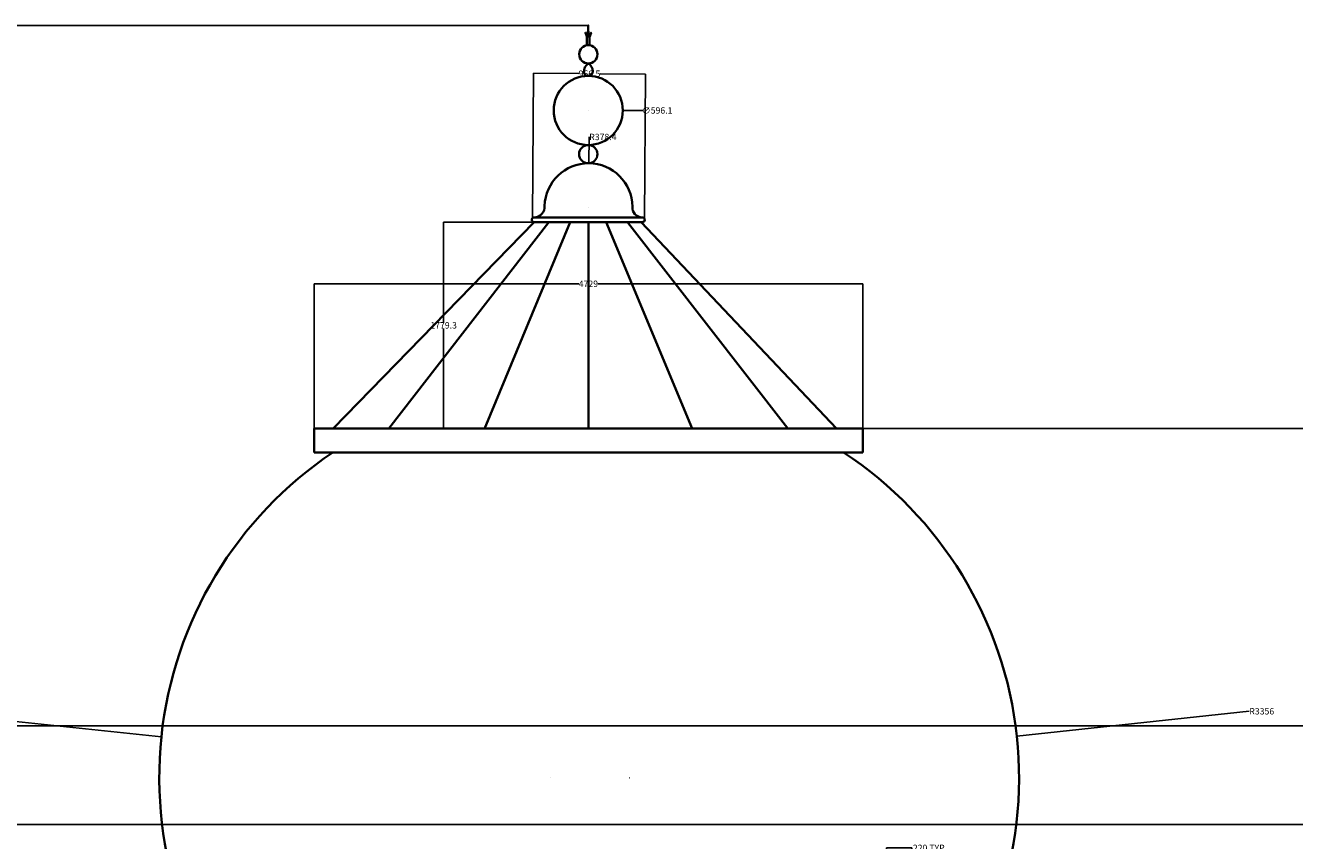
# Model space of a CAD drawing. Units: millimetres. Extents: x 8570 to 49085, y 3782 to 24863.
# Tile 10 of 15: x 17549 to 28488, y 17835 to 24863. Entities that reach past the tile are written whole.
import ezdxf

# ---------------------------------------------------------------- set-up
doc = ezdxf.new("R2010")
doc.units = ezdxf.units.MM
doc.header["$MEASUREMENT"] = 0
doc.header["$PDMODE"] = 3
doc.layers.add('A-ANNO-DIMS', color=2, linetype='Continuous', lineweight=18)
doc.layers.add('A-ROOF-DOME', color=7, linetype='Continuous', lineweight=35)
doc.styles.get("Standard").update_dxf_attribs({"font": 'arial.ttf'})
doc.dimstyles.get("Standard").update_dxf_attribs({"dimtxt": 55, "dimasz": 0.18, "dimexe": 0.18, "dimexo": 0.0625, "dimgap": 0.09, "dimtad": 0, "dimtih": 1, "dimtoh": 1, "dimdec": 0, "dimzin": 0, "dimdsep": 46, "dimtxsty": 'Standard', "dimcen": 0.09, "dimadec": 0, "dimazin": 0, "dimtfac": 1, "dimtdec": 0, "dimtofl": 0, "dimtmove": 0, "dimatfit": 3, "dimfxl": 1, "dimtolj": 1, "dimtzin": 0, "dimarcsym": 0})

# ---------------------------------------------------------------- blocks, each defined once
blk = doc.blocks.new('*D20')
at = {"layer": 'A-ANNO-DIMS', "color": 0, "lineweight": -2, "transparency": 16777216}
for p, q in [((24969, 16396.42408182047), (24969, 17772.62081909354)), ((24969.18, 17772.44081909354), (25188.82, 17772.44081909354)), ((25189, 16396.42408182047), (25189, 17772.62081909354)), ((25189, 17772.44081909354), (25189.18, 17772.44081909354))]:
    blk.add_line(p, q, dxfattribs=at)
at = {"layer": 'A-ANNO-DIMS', "color": 0, "transparency": 16777216}
for points in [[(24969.18, 17772.47081909354), (24969.18, 17772.41081909354), (24969, 17772.44081909354)], [(25188.82, 17772.47081909354), (25188.82, 17772.41081909354), (25189, 17772.44081909354)]]:
    blk.add_solid(points, dxfattribs=at)
at = {"layer": 'Defpoints', "color": 0, "transparency": 16777216}
for p in [(25189, 17772.44081909354), (24969, 16396.36158182047), (25189, 16396.36158182047)]:
    blk.add_point(p, dxfattribs=at)
at = {"layer": 'A-ANNO-DIMS', "color": 0, "transparency": 16777216, "insert": (25344.96577080491, 17772.44081909354), "char_height": 55, "attachment_point": 5}
blk.add_mtext('\\A1;220 TYP.', dxfattribs=at)
blk = doc.blocks.new('*D44')
at = {"layer": 'A-ANNO-DIMS', "color": 0, "lineweight": -2, "transparency": 16777216}
for p, q in [((22399.68750000001, 24862.95258900002), (8684.320000000003, 24862.95258900002)), ((8684.500000000005, 24862.77258900002), (8684.500000000005, 15410.3978088247)), ((8684.50000000001, 5901.680000000001), (8684.500000000005, 15354.05478017531)), ((10843.9375, 5901.500000000002), (8684.32000000001, 5901.500000000001))]:
    blk.add_line(p, q, dxfattribs=at)
at = {"layer": 'A-ANNO-DIMS', "color": 0, "transparency": 16777216}
for points in [[(8684.470000000005, 24862.77258900002), (8684.530000000006, 24862.77258900002), (8684.500000000005, 24862.95258900002)], [(8684.470000000008, 5901.680000000001), (8684.53000000001, 5901.680000000001), (8684.50000000001, 5901.500000000001)]]:
    blk.add_solid(points, dxfattribs=at)
at = {"layer": 'Defpoints', "color": 0, "transparency": 16777216}
for p in [(8684.500000000005, 24862.95258900002), (22399.75000000001, 24862.95258900002), (10844, 5901.500000000002)]:
    blk.add_point(p, dxfattribs=at)
at = {"layer": 'A-ANNO-DIMS', "color": 0, "transparency": 16777216, "insert": (8684.500000000013, 15382.2262945), "char_height": 55, "attachment_point": 5}
blk.add_mtext('\\A1;18961', dxfattribs=at)
blk = doc.blocks.new('*D54')
at = {"layer": 'A-ANNO-DIMS', "color": 0, "lineweight": -2, "transparency": 16777216}
for p, q in [((24765.69099400002, 21387.41061700001), (36055.18000000003, 21387.41061700001)), ((36055.00000000003, 21387.23061700001), (36055.00000000003, 19513.3036883513)), ((36055.00000000003, 17582.996214), (36055.00000000003, 19456.92314264871)), ((26017.61772600001, 17582.816214), (36055.18000000003, 17582.816214))]:
    blk.add_line(p, q, dxfattribs=at)
at = {"layer": 'A-ANNO-DIMS', "color": 0, "transparency": 16777216}
for points in [[(36054.97000000003, 21387.23061700001), (36055.03000000003, 21387.23061700001), (36055.00000000003, 21387.41061700001)], [(36054.97000000003, 17582.996214), (36055.03000000003, 17582.996214), (36055.00000000003, 17582.816214)]]:
    blk.add_solid(points, dxfattribs=at)
at = {"layer": 'Defpoints', "color": 0, "transparency": 16777216}
for p in [(24765.62849400002, 21387.41061700001), (36055.00000000003, 21387.41061700001), (26017.55522600002, 17582.816214)]:
    blk.add_point(p, dxfattribs=at)
at = {"layer": 'A-ANNO-DIMS', "color": 0, "transparency": 16777216, "insert": (36055.00000000003, 19485.11341549999), "char_height": 55, "attachment_point": 5}
blk.add_mtext('\\A1;3804.6', dxfattribs=at)
blk = doc.blocks.new('*D55')
at = {"layer": 'A-ANNO-DIMS', "color": 0, "lineweight": -2, "transparency": 16777216}
for p, q in [((20036.761255, 21387.473117), (20036.761255, 22635.590617)), ((20036.941255, 22635.410617), (22317.81701638268, 22635.410617)), ((24765.448494, 22635.410617), (22484.57273261732, 22635.410617)), ((24765.628494, 21387.473117), (24765.628494, 22635.590617))]:
    blk.add_line(p, q, dxfattribs=at)
at = {"layer": 'A-ANNO-DIMS', "color": 0, "transparency": 16777216}
for points in [[(20036.941255, 22635.440617), (20036.941255, 22635.380617), (20036.761255, 22635.410617)], [(24765.448494, 22635.440617), (24765.448494, 22635.380617), (24765.628494, 22635.410617)]]:
    blk.add_solid(points, dxfattribs=at)
at = {"layer": 'Defpoints', "color": 0, "transparency": 16777216}
for p in [(24765.628494, 22635.410617), (20036.761255, 21387.410617), (24765.628494, 21387.410617)]:
    blk.add_point(p, dxfattribs=at)
at = {"layer": 'A-ANNO-DIMS', "color": 0, "transparency": 16777216, "insert": (22401.1948745, 22635.410617), "char_height": 55, "attachment_point": 5}
blk.add_mtext('\\A1;4729', dxfattribs=at)
blk = doc.blocks.new('*D56')
at = {"layer": 'A-ANNO-DIMS', "color": 0, "lineweight": -2, "transparency": 16777216}
for p, q in [((21918.71662826998, 23201.96913155994), (21927.18924882475, 24450.05787384567)), ((21927.36802277985, 24449.8766560955), (22317.33882302958, 24447.22934865172)), ((22893.49917307467, 24443.31809790548), (22503.52837282495, 24445.96540534927)), ((22885.20777026998, 23195.40812955994), (22893.68039082485, 24443.49687186058))]:
    blk.add_line(p, q, dxfattribs=at)
at = {"layer": 'A-ANNO-DIMS', "color": 0, "transparency": 16777216}
for points in [[(21927.36822642944, 24449.90665540428), (21927.36781913026, 24449.84665678673), (21927.18802692721, 24449.87787799304)], [(22893.49937672426, 24443.34809721426), (22893.49896942508, 24443.28809859671), (22893.67916892731, 24443.31687600795)]]:
    blk.add_solid(points, dxfattribs=at)
at = {"layer": 'Defpoints', "color": 0, "transparency": 16777216}
for p in [(22893.67916892731, 24443.31687600795), (21918.716204, 23201.906633), (22885.207346, 23195.345631)]:
    blk.add_point(p, dxfattribs=at)
at = {"layer": 'A-ANNO-DIMS', "color": 0, "transparency": 16777216, "insert": (22410.43359792727, 24446.5973770005), "char_height": 55, "attachment_point": 5}
blk.add_mtext('\\A1;966.5', dxfattribs=at)
blk = doc.blocks.new('*D57')
at = {"layer": 'A-ANNO-DIMS', "color": 0, "lineweight": -2, "transparency": 16777216}
for p, q in [((22401.13237400001, 23166.67013700001), (21153.01487400002, 23166.67013700001)), ((21153.19487400002, 23166.49013700001), (21153.19487400002, 22305.23064985131)), ((21153.19487400002, 21387.59061700001), (21153.19487400002, 22248.85010414871)), ((22401.13237400001, 21387.41061700001), (21153.01487400002, 21387.41061700001))]:
    blk.add_line(p, q, dxfattribs=at)
at = {"layer": 'A-ANNO-DIMS', "color": 0, "transparency": 16777216}
for points in [[(21153.16487400002, 23166.49013700001), (21153.22487400002, 23166.49013700001), (21153.19487400002, 23166.67013700001)], [(21153.16487400002, 21387.59061700001), (21153.22487400002, 21387.59061700001), (21153.19487400002, 21387.41061700001)]]:
    blk.add_solid(points, dxfattribs=at)
at = {"layer": 'Defpoints', "color": 0, "transparency": 16777216}
for p in [(21153.19487400002, 23166.67013700001), (22401.19487400001, 23166.67013700001), (22401.19487400001, 21387.41061700001)]:
    blk.add_point(p, dxfattribs=at)
at = {"layer": 'A-ANNO-DIMS', "color": 0, "transparency": 16777216, "insert": (21153.19487400002, 22277.040377), "char_height": 55, "attachment_point": 5}
blk.add_mtext('\\A1;1779.3', dxfattribs=at)
blk = doc.blocks.new('*D61')
at = {"layer": 'A-ANNO-DIMS', "color": 0, "lineweight": -2, "transparency": 16777216}
for p, q in [((33091.43750000002, 17974), (8684.320000000003, 17974)), ((8684.500000000005, 17973.82), (8684.500000000005, 15935.4402728513)), ((8684.500000000005, 13840.68), (8684.500000000005, 15879.0597271487)), ((33041.43750000001, 13840.50000000001), (8684.320000000003, 13840.5))]:
    blk.add_line(p, q, dxfattribs=at)
at = {"layer": 'A-ANNO-DIMS', "color": 0, "transparency": 16777216}
for points in [[(8684.470000000008, 17973.82), (8684.530000000006, 17973.82), (8684.500000000005, 17974)], [(8684.470000000008, 13840.68), (8684.530000000006, 13840.68), (8684.500000000005, 13840.5)]]:
    blk.add_solid(points, dxfattribs=at)
at = {"layer": 'Defpoints', "color": 0, "transparency": 16777216}
for p in [(8684.500000000005, 17974), (33091.50000000002, 17974), (33041.50000000002, 13840.50000000001)]:
    blk.add_point(p, dxfattribs=at)
at = {"layer": 'A-ANNO-DIMS', "color": 0, "transparency": 16777216, "insert": (8684.500000000013, 15907.24999999999), "char_height": 55, "attachment_point": 5}
blk.add_mtext('\\A1;4133.5', dxfattribs=at)
blk = doc.blocks.new('*D62')
at = {"layer": 'A-ANNO-DIMS', "color": 0, "lineweight": -2, "transparency": 16777216}
for p, q in [((33128.43750000002, 18823.5), (8684.320000000003, 18823.5)), ((8684.500000000005, 18823.32), (8684.500000000005, 18426.9215143247)), ((8684.500000000005, 17974.18), (8684.500000000005, 18370.57848567531)), ((33091.43750000002, 17974), (8684.320000000003, 17974))]:
    blk.add_line(p, q, dxfattribs=at)
at = {"layer": 'A-ANNO-DIMS', "color": 0, "transparency": 16777216}
for points in [[(8684.470000000008, 18823.32), (8684.530000000006, 18823.32), (8684.500000000005, 18823.5)], [(8684.470000000008, 17974.18), (8684.530000000006, 17974.18), (8684.500000000005, 17974)]]:
    blk.add_solid(points, dxfattribs=at)
at = {"layer": 'Defpoints', "color": 0, "transparency": 16777216}
for p in [(8684.500000000005, 18823.5), (33128.50000000001, 18823.5), (33091.50000000002, 17974)]:
    blk.add_point(p, dxfattribs=at)
at = {"layer": 'A-ANNO-DIMS', "color": 0, "transparency": 16777216, "insert": (8684.500000000013, 18398.74999999999), "char_height": 55, "attachment_point": 5}
blk.add_mtext('\\A1;849.5', dxfattribs=at)
blk = doc.blocks.new('*D79')
at = {"layer": 'A-ANNO-DIMS', "color": 0, "lineweight": -2, "transparency": 16777216}
for p, q in [((16711.08233114532, 18940.57169344747), (18720.56133109179, 18730.77165433857)), ((22070.080402, 18381.055079), (22070.260402, 18381.055079)), ((22070.170402, 18380.965079), (22070.170402, 18381.145079))]:
    blk.add_line(p, q, dxfattribs=at)
at = {"layer": 'A-ANNO-DIMS', "color": 0, "transparency": 16777216}
blk.add_solid([(18720.56444631488, 18730.80149215661), (18720.55821586869, 18730.74181652054), (18720.740358, 18730.752963)], dxfattribs=at)
at = {"layer": 'Defpoints', "color": 0, "transparency": 16777216}
for p in [(18720.740358, 18730.752963), (22070.170402, 18381.055079)]:
    blk.add_point(p, dxfattribs=at)
at = {"layer": 'A-ANNO-DIMS', "color": 0, "transparency": 16777216, "insert": (16570.52848394205, 18940.57169344747), "char_height": 55, "attachment_point": 5}
blk.add_mtext('\\A1;R3367.6', dxfattribs=at)
blk = doc.blocks.new('*D80')
at = {"layer": 'A-ANNO-DIMS', "color": 0, "lineweight": -2, "transparency": 16777216}
for p, q in [((28095.78462736095, 18950.21251423877), (26093.79075351863, 18735.17220077332)), ((22756.567043, 18376.720415), (22756.747043, 18376.720415)), ((22756.657043, 18376.630415), (22756.657043, 18376.810415))]:
    blk.add_line(p, q, dxfattribs=at)
at = {"layer": 'A-ANNO-DIMS', "color": 0, "transparency": 16777216}
blk.add_solid([(26093.78754955641, 18735.20202919309), (26093.79395748085, 18735.14237235355), (26093.611783, 18735.152977)], dxfattribs=at)
at = {"layer": 'Defpoints', "color": 0, "transparency": 16777216}
for p in [(26093.611783, 18735.152977), (22756.657043, 18376.720415)]:
    blk.add_point(p, dxfattribs=at)
at = {"layer": 'A-ANNO-DIMS', "color": 0, "transparency": 16777216, "insert": (28204.2989111263, 18950.21251423877), "char_height": 55, "attachment_point": 5}
blk.add_mtext('\\A1;R3356', dxfattribs=at)
blk = doc.blocks.new('*D85')
at = {"layer": 'A-ANNO-DIMS', "color": 0, "lineweight": -2, "transparency": 16777216}
for p, q in [((22399.65999999999, 24129.78207699999), (22399.83999999999, 24129.78207699999)), ((22399.74999999999, 24129.69207699999), (22399.74999999999, 24129.87207699999)), ((22876.64108959999, 24129.7819538), (22697.986931, 24129.78199995349))]:
    blk.add_line(p, q, dxfattribs=at)
at = {"layer": 'A-ANNO-DIMS', "color": 0, "transparency": 16777216}
blk.add_solid([(22697.98693100775, 24129.81199995349), (22697.98693099225, 24129.75199995349), (22697.806931, 24129.78199999999)], dxfattribs=at)
at = {"layer": 'Defpoints', "color": 0, "transparency": 16777216}
for p in [(22101.69306899999, 24129.78215399999), (22697.806931, 24129.78199999999)]:
    blk.add_point(p, dxfattribs=at)
at = {"layer": 'A-ANNO-DIMS', "color": 0, "transparency": 16777216, "insert": (22994.14070760818, 24129.7819538), "char_height": 55, "attachment_point": 5}
blk.add_mtext('\\A1;∅596.1', dxfattribs=at)
blk = doc.blocks.new('*D86')
at = {"layer": 'A-ANNO-DIMS', "color": 0, "lineweight": -2, "transparency": 16777216}
for p, q in [((22406.58913879506, 23901.07551755377), (22404.85637372993, 23674.20287275025)), ((22406.76913879506, 23901.07551755377), (22406.58913879506, 23901.07551755377)), ((22401.874766, 23295.60181100001), (22402.054766, 23295.60181100001)), ((22401.964766, 23295.51181100001), (22401.964766, 23295.691811))]:
    blk.add_line(p, q, dxfattribs=at)
at = {"layer": 'A-ANNO-DIMS', "color": 0, "transparency": 16777216}
blk.add_solid([(22404.82637460489, 23674.20310187191), (22404.88637285497, 23674.2026436286), (22404.854999, 23674.022878)], dxfattribs=at)
at = {"layer": 'Defpoints', "color": 0, "transparency": 16777216}
for p in [(22404.854999, 23674.022878), (22401.964766, 23295.601811)]:
    blk.add_point(p, dxfattribs=at)
at = {"layer": 'A-ANNO-DIMS', "color": 0, "transparency": 16777216, "insert": (22525.8632315645, 23901.07551755377), "char_height": 55, "attachment_point": 5}
blk.add_mtext('\\A1;R378.4', dxfattribs=at)

msp = doc.modelspace()

# ---------------------------------------------------------------- linework, layer by layer
at = {"layer": 'A-ROOF-DOME'}
for p, q in [((21933.31163890215, 23207.95226036421), (22866.18836109828, 23207.95226036421)), ((20680.34955918219, 21387.41061714557), (22061.23658788237, 23166.67013693519)), ((22245.17052051611, 23166.47437941175), (21506.40556353246, 21386.27981236571)), ((21933.31163890215, 23166.67013693519), (22866.18836109828, 23166.67013693519)), ((22401.19487432002, 21387.41061714557), (22401.19487432001, 23166.67013693519)), ((22554.97078409327, 23166.67013693519), (23295.9848996439, 21387.41061714557)), ((24119.15044081824, 21387.41061714557), (22738.26341211805, 23166.67013693519)), ((24765.62849371602, 21387.41061714557), (20036.76125492401, 21387.41061714557)), ((20201.88974864003, 21387.41061714557), (20036.76125492401, 21387.41061714557)), ((20036.76125492401, 21387.41061714557), (20036.76125492401, 21181.00000000008)), ((24765.62849371602, 21181.00000000056), (24765.62849371602, 21387.41061714557)), ((20036.76125492401, 21181.00000000008), (20199, 21181.00000000009)), ((20199, 21181.00000000009), (24600.5, 21181.00000000056)), ((24600.5, 21181.00000000056), (24765.62849371602, 21181.00000000056))]:
    msp.add_line(p, q, dxfattribs=at)
for points in [[(22397.34097207832, 24769.1925821318), (22399.75000000021, 24862.95258863299), (22402.48961008092, 24770.18272427195)], [(22389.90887414118, 24761.41097521227), (22374.72803576594, 24799.11951502219), (22399.52226019253, 24766.30577158642)], [(22411.26633617924, 24754.7145213354), (22411.26633617924, 24692.89699852589), (22387.7781842058, 24692.89699852589), (22387.7781842058, 24754.7145213354)], [(22409.10514092229, 24761.35151888434), (22424.51927405761, 24798.96529731802), (22399.52226019253, 24766.30577158642)], [(20201.88974864003, 21387.41061714557), (21933.31163890215, 23166.67013693519)], [(24538.57681485692, 21387.41061714557), (22856.74310635929, 23166.67013693519)]]:
    msp.add_lwpolyline(points, dxfattribs=at)
for points in [[(22439.79842726564, 24468.86954000115, 0.2163087324469712), (22400.41987042385, 24535.20213256301, 0.244698442998971), (22360.76532962731, 24458.67890765262, 0.244698442998971)], [(21933.31163890215, 23207.95226036421, 0.4376812219515575), (22023.66985556199, 23305.79089289094, -0.9808935761650767), (22780.37117801563, 23300.01139561088, 0.4496045632983121), (22866.18836109828, 23207.95226036421, 0.9757223232571062)]]:
    msp.add_lwpolyline(points, format="xyb", dxfattribs=at)
for centre, radius in [((22400.4198704239, 24614.05098831234), 78.84885574933196), ((22399.75000000021, 24129.78207653386), 298.0569311574765), ((22399.75000000021, 23752.87628962706), 78.84885574933196)]:
    msp.add_circle(centre, radius, dxfattribs=at)
for centre, radius, start, end in [((22399.52226019253, 24754.56068812834), 11.74508345808496, 0.7504625718552804, 179.2495374281447), ((22399.75000000025, 24467.89918876868), 40.06018107730136, 193.306535650578, 1.387973465606026), ((21933.31163890215, 23187.3111986497), 20.64106171450211, 90, 270), ((22866.18836109828, 23187.3111986497), 20.64106171450211, 270, 90), ((22070.1704024526, 18381.05507927042), 3367.635703892862, 123.7543431943301, 224.3248907677251), ((22756.65704265762, 18376.72041492595), 3356.14970503511, 315.5869641412231, 56.67466470512833)]:
    msp.add_arc(centre, radius, start, end, dxfattribs=at)

# ---------------------------------------------------------------- dimensions: what is measured, and where the dimension line sits
at = {"layer": 'A-ANNO-DIMS'}
for base, p1, p2, angle, override, picture, middle in [((8684.500000000005, 24862.95258900002), (10844, 5901.5), (22399.75, 24862.952589), 90, {"dimdec": 0, "dimlfac": 1, "dimrnd": 0, "dimzin": 0, "dimdsep": 46, "dimlunit": 2}, '*D44', (8684.500000000013, 15382.2262945)), ((22893.67916892731, 24443.31687600795), (21918.716204, 23201.906633), (22885.207346, 23195.345631), 359.6110549466791, {"dimdec": 1, "dimlfac": 1, "dimrnd": 0, "dimzin": 0, "dimdsep": 46, "dimlunit": 2}, '*D56', (22410.43359792727, 24446.5973770005)), ((21153.19487400002, 23166.67013700001), (22401.194874, 21387.410617), (22401.194874, 23166.670137), 90.00000000000036, {"dimdec": 1, "dimlfac": 1, "dimrnd": 0, "dimzin": 0, "dimdsep": 46, "dimlunit": 2}, '*D57', (21153.19487400002, 22277.040377)), ((36055.00000000003, 21387.41061700001), (26017.555226, 17582.816214), (24765.628494, 21387.410617), 90, {"dimdec": 1, "dimlfac": 1, "dimrnd": 0, "dimzin": 0, "dimdsep": 46, "dimlunit": 2}, '*D54', (36055.00000000003, 19485.11341549999)), ((8684.500000000005, 18823.5), (33091.5, 17974), (33128.5, 18823.5), 90, {"dimdec": 1, "dimlfac": 1, "dimrnd": 0, "dimzin": 0, "dimdsep": 46, "dimlunit": 2}, '*D62', (8684.500000000013, 18398.74999999999)), ((8684.500000000005, 17974), (33041.5, 13840.5), (33091.5, 17974), 90, {"dimdec": 1, "dimlfac": 1, "dimrnd": 0, "dimzin": 0, "dimdsep": 46, "dimlunit": 2}, '*D61', (8684.500000000013, 15907.24999999999))]:
    dim = msp.add_linear_dim(base=base, p1=p1, p2=p2, angle=angle, dimstyle='Standard', override=override, dxfattribs=at)
    dim.commit()
    dim.dimension.update_dxf_attribs({"geometry": picture, "text_midpoint": middle})
dim = msp.add_diameter_dim_2p(p1=(22101.69306899999, 24129.78215399999), p2=(22697.806931, 24129.78199999999), dimstyle='Standard', override={"dimdec": 1, "dimlfac": 1, "dimrnd": 0, "dimzin": 0, "dimdsep": 46, "dimlunit": 2}, dxfattribs=at)
dim.commit()
dim.dimension.update_dxf_attribs({"geometry": '*D85', "text_midpoint": (22876.64108959999, 24129.7819538), "dimtype": 163})
for center, mpoint, override, picture, middle in [((22401.964766, 23295.601811), (22404.854999, 23674.022878), {"dimdec": 1, "dimlfac": 1, "dimrnd": 0, "dimzin": 0, "dimdsep": 46, "dimlunit": 2}, '*D86', (22525.8632315645, 23901.07551755377)), ((22070.170402, 18381.055079), (18720.740358, 18730.752963), {"dimdec": 1, "dimlfac": 1, "dimrnd": 0, "dimzin": 0, "dimdsep": 46, "dimlunit": 2}, '*D79', (16711.08233114532, 18940.57169344747)), ((22756.657043, 18376.720415), (26093.611783, 18735.152977), {"dimdec": 0, "dimlfac": 1, "dimrnd": 0, "dimzin": 0, "dimdsep": 46, "dimlunit": 2}, '*D80', (28095.78462736095, 18950.21251423877))]:
    dim = msp.add_radius_dim(center=center, mpoint=mpoint, dimstyle='Standard', override=override, dxfattribs=at)
    dim.commit()
    dim.dimension.update_dxf_attribs({"geometry": picture, "text_midpoint": middle, "dimtype": 164})
dim = msp.add_linear_dim(base=(24765.628494, 22635.410617), p1=(20036.761255, 21387.410617), p2=(24765.628494, 21387.410617), dimstyle='Standard', override={"dimdec": 0, "dimlfac": 1, "dimrnd": 0, "dimzin": 0, "dimdsep": 46, "dimlunit": 2}, dxfattribs=at)
dim.commit()
dim.dimension.update_dxf_attribs({"geometry": '*D55', "text_midpoint": (22401.1948745, 22635.410617)})
dim = msp.add_linear_dim(base=(25189, 17772.44081909354), p1=(24969, 16396.36158182047), p2=(25189, 16396.36158182047), text='<> TYP.', dimstyle='Standard', override={"dimdec": 0, "dimlfac": 1, "dimrnd": 0, "dimzin": 0, "dimdsep": 46, "dimlunit": 2}, dxfattribs=at)
dim.commit()
dim.dimension.update_dxf_attribs({"geometry": '*D20', "text_midpoint": (25344.96577080491, 17772.44081909354)})

doc.saveas('drawing.dxf')
